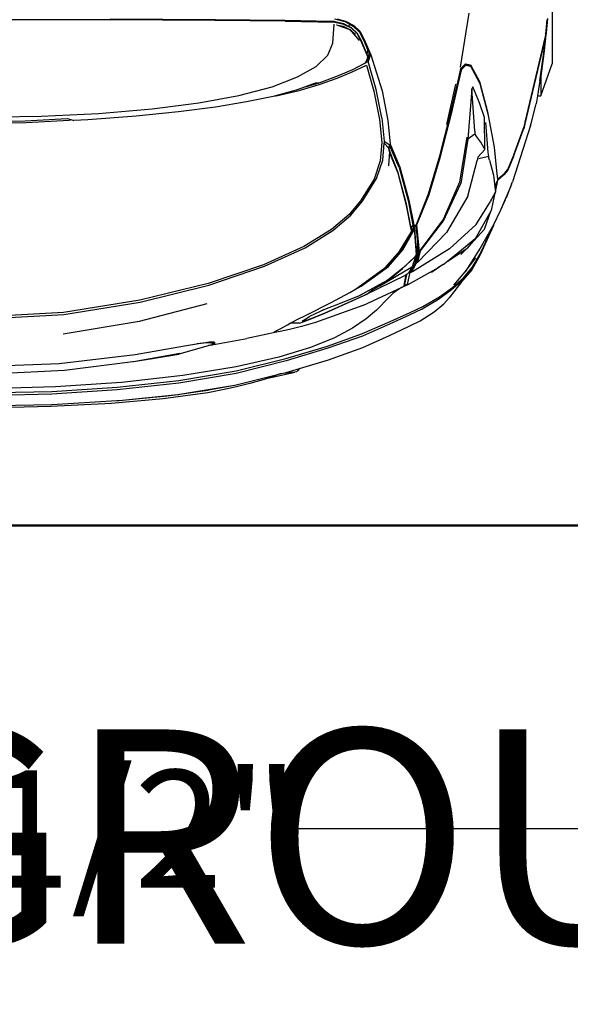
# Model space of a CAD drawing. Units: inches. Extents: x 22042254 to 25404563, y 17568978 to 17626777.
# Tile 23 of 45: x 22179852 to 22179889, y 17626160 to 17626227. Entities that reach past the tile are written whole.
import ezdxf

# ---------------------------------------------------------------- set-up
doc = ezdxf.new("R2010")
doc.units = ezdxf.units.IN
doc.header["$MEASUREMENT"] = 0
for name, color, linetype, lineweight in [('A-ANNO-DIMS', 2, 'Continuous', 18), ('A-SITE-VEHI', 8, 'Continuous', 18), ('text', 7, 'Continuous', 25), ('walls', 252, 'Continuous', 50)]:
    doc.layers.add(name, color=color, linetype=linetype, lineweight=lineweight)
doc.layers.add('Edges', color=250, linetype='Continuous')
doc.styles.get("Standard").update_dxf_attribs({"font": 'arial.ttf'})
doc.dimstyles.get("Standard").update_dxf_attribs({"dimtxt": 8, "dimasz": 0.18, "dimexe": 0.18, "dimexo": 0.0625, "dimgap": 0.09, "dimtad": 0, "dimtih": 1, "dimtoh": 1, "dimzin": 0, "dimdsep": 46, "dimlunit": 3, "dimtxsty": 'Standard', "dimcen": 0.09, "dimadec": 0, "dimazin": 0, "dimtfac": 1, "dimtofl": 0, "dimtmove": 0, "dimatfit": 3, "dimfxl": 1, "dimtolj": 1, "dimtzin": 0, "dimarcsym": 0})

# ---------------------------------------------------------------- blocks, each defined once
blk = doc.blocks.new('Nissan Qashqai pl')
at = {"layer": 'Edges'}
for p, q in [((10.9577, 12.8101), (11.1283, 12.8101)), ((11.0576, 12.8026), (11.0798, 12.8008)), ((11.0768, 12.8008), (11.059, 12.8023)), ((11.0811, 12.8004), (11.0768, 12.8008)), ((11.0798, 12.8008), (11.0872, 12.7999)), ((11.0827, 12.8001), (11.0811, 12.8004)), ((11.0827, 12.8001), (11.0813, 12.7998)), ((11.0836, 12.8002), (11.0827, 12.8001)), ((11.0856, 12.7994), (11.0827, 12.8001)), ((11.0872, 12.7999), (11.0836, 12.8002)), ((11.0836, 12.8002), (11.0882, 12.7992)), ((11.2196, 12.7681), (11.0856, 12.7994)), ((11.0883, 12.7998), (11.0872, 12.7999)), ((11.0882, 12.7992), (11.2222, 12.7676)), ((11.0883, 12.7998), (11.1123, 12.797)), ((11.1147, 12.7965), (11.0883, 12.7998)), ((11.1123, 12.797), (11.1475, 12.7921)), ((11.1547, 12.791), (11.1147, 12.7965)), ((11.1783, 12.7921), (11.1283, 12.8101)), ((11.1475, 12.7921), (11.1525, 12.7914)), ((11.1475, 12.7921), (11.1783, 12.7921)), ((11.1525, 12.7914), (11.1547, 12.791)), ((11.1547, 12.791), (11.1783, 12.787)), ((11.1783, 12.787), (11.1783, 12.7921)), ((11.1783, 12.787), (11.1906, 12.7849)), ((11.1906, 12.7849), (11.1909, 12.7849)), ((11.193, 12.7845), (11.1909, 12.7849)), ((11.2215, 12.7775), (11.193, 12.7845)), ((11.2247, 12.767), (11.2163, 12.7689)), ((11.22, 12.768), (11.2196, 12.7681)), ((11.2247, 12.767), (11.22, 12.768)), ((11.2247, 12.7764), (11.2215, 12.7775)), ((11.2222, 12.7676), (11.2271, 12.7664)), ((11.2247, 12.7764), (11.3124, 12.7479)), ((11.2253, 12.7668), (11.2247, 12.767)), ((11.2304, 12.7649), (11.2253, 12.7668)), ((11.2253, 12.7668), (11.2271, 12.7664)), ((11.2271, 12.7664), (11.2296, 12.7658)), ((11.2271, 12.7664), (11.2277, 12.7662)), ((11.2277, 12.7662), (11.2296, 12.7658)), ((11.2732, 12.7496), (11.2277, 12.7662)), ((11.2704, 12.7504), (11.2304, 12.7649)), ((11.2702, 12.7507), (11.2704, 12.7504)), ((11.2704, 12.7506), (11.2707, 12.7503)), ((11.2707, 12.7503), (11.2704, 12.7504)), ((11.2719, 12.7498), (11.2707, 12.7503)), ((11.2934, 12.741), (11.2719, 12.7498)), ((11.2732, 12.7496), (11.2946, 12.7409)), ((11.3, 12.735), (11.2934, 12.741)), ((11.2946, 12.7409), (11.3018, 12.7346)), ((11.3081, 12.7253), (11.3, 12.735)), ((11.3018, 12.7346), (11.3103, 12.7249)), ((11.3161, 12.7467), (11.3124, 12.7479)), ((11.3161, 12.7467), (11.3376, 12.7381)), ((11.3192, 12.7454), (11.3566, 12.7294)), ((11.3405, 12.7369), (11.3376, 12.7381)), ((11.3405, 12.7369), (11.3566, 12.7294)), ((11.2091, 12.7103), (11.2583, 12.7196)), ((11.2583, 12.7196), (11.2956, 12.7234)), ((11.2956, 12.7234), (11.3085, 12.7247)), ((11.3022, 12.7186), (11.3252, 12.7213)), ((11.3086, 12.7247), (11.3081, 12.7253)), ((11.3081, 12.7253), (11.3087, 12.7247)), ((11.3085, 12.7247), (11.3086, 12.7247)), ((11.3086, 12.7247), (11.3087, 12.7247)), ((11.3087, 12.7247), (11.3103, 12.7249)), ((11.3103, 12.7249), (11.3103, 12.7249)), ((11.3103, 12.7249), (11.3106, 12.7249)), ((11.3106, 12.7249), (11.314, 12.7238)), ((11.317, 12.7227), (11.3119, 12.7236)), ((11.3132, 12.7243), (11.3256, 12.7215)), ((11.314, 12.7238), (11.317, 12.7227)), ((11.314, 12.7238), (11.3242, 12.7216)), ((11.3242, 12.7216), (11.317, 12.7227)), ((11.3198, 12.7211), (11.3252, 12.7213)), ((11.3242, 12.7216), (11.3256, 12.7215)), ((11.3252, 12.7213), (11.3283, 12.7214)), ((11.3256, 12.7215), (11.3283, 12.7214)), ((11.3283, 12.7214), (11.3297, 12.7206)), ((11.3297, 12.7206), (11.3446, 12.7173)), ((11.3297, 12.7206), (11.3302, 12.7203)), ((11.3302, 12.7203), (11.3446, 12.7173)), ((11.3302, 12.7203), (11.3394, 12.7152)), ((11.3566, 12.7294), (11.3796, 12.7187)), ((11.3796, 12.7187), (11.4164, 12.6974)), ((11.3796, 12.7187), (11.3807, 12.7182)), ((11.156, 12.6966), (11.203, 12.7093)), ((11.1589, 12.6971), (11.2062, 12.7098)), ((11.2121, 12.7043), (11.189, 12.6968)), ((11.203, 12.7093), (11.2091, 12.7103)), ((11.2062, 12.7098), (11.2091, 12.7103)), ((11.2622, 12.7051), (11.2121, 12.7043)), ((11.2199, 12.706), (11.2666, 12.7097)), ((11.2601, 12.7037), (11.2505, 12.6987)), ((11.2622, 12.7051), (11.2601, 12.7037)), ((11.2743, 12.6942), (11.2622, 12.7051)), ((11.2666, 12.7097), (11.2729, 12.7104)), ((11.2787, 12.7123), (11.2729, 12.7104)), ((11.2729, 12.7104), (11.2766, 12.6957)), ((11.2787, 12.7123), (11.3022, 12.7186)), ((11.3394, 12.7152), (11.3434, 12.7138)), ((11.3394, 12.7152), (11.342, 12.7137)), ((11.379, 12.6915), (11.3434, 12.7138)), ((11.3446, 12.7173), (11.3571, 12.7146)), ((11.3583, 12.7142), (11.3571, 12.7146)), ((11.3571, 12.7146), (11.3821, 12.7008)), ((11.3583, 12.7142), (11.3821, 12.7008)), ((11.3864, 12.7044), (11.3583, 12.7142)), ((11.3807, 12.7182), (11.4267, 12.6979)), ((11.4228, 12.6989), (11.3807, 12.7182)), ((11.4163, 12.6775), (11.3864, 12.7044)), ((11.1298, 12.6823), (11.156, 12.6966)), ((11.1365, 12.6851), (11.1589, 12.6971)), ((11.189, 12.6968), (11.1644, 12.6862)), ((11.2337, 12.6892), (11.1672, 12.6844)), ((11.2337, 12.6892), (11.2382, 12.6892)), ((11.2382, 12.6892), (11.2401, 12.6908)), ((11.2382, 12.6892), (11.2459, 12.6785)), ((11.2505, 12.6987), (11.2401, 12.6908)), ((11.2743, 12.6942), (11.2791, 12.6927)), ((11.335, 12.6786), (11.2791, 12.6927)), ((11.379, 12.6915), (11.417, 12.6499)), ((11.3821, 12.7008), (11.4014, 12.69)), ((11.4014, 12.69), (11.4022, 12.6894)), ((11.4014, 12.69), (11.4265, 12.6594)), ((11.4022, 12.6894), (11.4163, 12.6775)), ((11.4022, 12.6894), (11.4265, 12.6594)), ((11.4164, 12.6974), (11.4531, 12.6744)), ((11.4243, 12.6982), (11.4228, 12.6989)), ((11.4464, 12.6853), (11.4243, 12.6982)), ((11.4267, 12.6979), (11.4498, 12.6844)), ((11.4531, 12.6744), (11.4314, 12.6911)), ((11.1336, 12.667), (11.0492, 12.6807)), ((11.1285, 12.6745), (11.1298, 12.6823)), ((11.1293, 12.6736), (11.1285, 12.6745)), ((11.1306, 12.6812), (11.1293, 12.6736)), ((11.1353, 12.6677), (11.1293, 12.6736)), ((11.1306, 12.6752), (11.1319, 12.6827)), ((11.1319, 12.6827), (11.1306, 12.6812)), ((11.1347, 12.671), (11.1306, 12.6752)), ((11.1319, 12.6827), (11.1365, 12.6851)), ((11.1644, 12.6862), (11.1672, 12.6844)), ((11.1672, 12.6844), (11.2459, 12.6785)), ((11.2428, 12.6769), (11.3132, 12.6652)), ((11.2459, 12.6785), (11.3153, 12.6672)), ((11.335, 12.6786), (11.3915, 12.6453)), ((11.4366, 12.6471), (11.4163, 12.6775)), ((11.4163, 12.6775), (11.4259, 12.6674)), ((11.4624, 12.6717), (11.4464, 12.6853)), ((11.4498, 12.6844), (11.4662, 12.6706)), ((11.4681, 12.6691), (11.4498, 12.6844)), ((11.4742, 12.6567), (11.4531, 12.6744)), ((11.1366, 12.6691), (11.1347, 12.671)), ((11.1358, 12.6676), (11.1353, 12.6677)), ((11.1358, 12.6676), (11.1366, 12.6691)), ((11.148, 12.665), (11.1358, 12.6676)), ((11.1401, 12.6682), (11.1366, 12.6691)), ((11.2066, 12.6527), (11.1401, 12.6682)), ((11.2063, 12.6515), (11.148, 12.665)), ((11.2232, 12.6458), (11.1598, 12.6594)), ((11.3132, 12.6652), (11.3715, 12.6398)), ((11.3733, 12.6404), (11.3153, 12.6672)), ((11.4265, 12.6594), (11.4366, 12.6471)), ((11.4774, 12.6543), (11.4624, 12.6717)), ((11.4662, 12.6706), (11.4815, 12.6531)), ((11.4681, 12.6691), (11.4936, 12.6491)), ((11.272, 12.6349), (11.2063, 12.6515)), ((11.2728, 12.6357), (11.2066, 12.6527)), ((11.3915, 12.6453), (11.4381, 12.6002)), ((11.417, 12.6499), (11.4529, 12.5922)), ((11.4366, 12.6471), (11.4408, 12.6419)), ((11.4408, 12.6419), (11.4411, 12.6414)), ((11.4924, 12.6339), (11.4774, 12.6543)), ((11.4815, 12.6531), (11.4963, 12.6328)), ((11.4936, 12.6491), (11.5033, 12.6408)), ((11.3311, 12.6172), (11.272, 12.6349)), ((11.3323, 12.6178), (11.2728, 12.6357)), ((11.3715, 12.6398), (11.4177, 12.6052)), ((11.4203, 12.6044), (11.3733, 12.6404)), ((11.4411, 12.6414), (11.4411, 12.6414)), ((11.4414, 12.6409), (11.4411, 12.6414)), ((11.4414, 12.6409), (11.447, 12.6315)), ((11.4455, 12.6336), (11.4414, 12.6409)), ((11.447, 12.6315), (11.4455, 12.6336)), ((11.4455, 12.6336), (11.4462, 12.6324)), ((11.447, 12.6315), (11.4462, 12.6324)), ((11.4732, 12.585), (11.4462, 12.6324)), ((11.447, 12.6315), (11.447, 12.6314)), ((11.4536, 12.6215), (11.447, 12.6314)), ((11.5074, 12.608), (11.4924, 12.6339)), ((11.4964, 12.6326), (11.4963, 12.6328)), ((11.4964, 12.6326), (11.5113, 12.6069)), ((11.5158, 12.6256), (11.5033, 12.6408)), ((11.3751, 12.5999), (11.3311, 12.6172)), ((11.3747, 12.6011), (11.3323, 12.6178)), ((11.5295, 12.6041), (11.5158, 12.6256)), ((11.38, 12.5988), (11.3747, 12.6011)), ((11.3751, 12.5999), (11.3762, 12.5999)), ((11.3752, 12.5998), (11.3751, 12.5999)), ((11.3763, 12.5998), (11.3752, 12.5998)), ((11.3764, 12.5993), (11.3752, 12.5998)), ((11.3792, 12.5982), (11.3764, 12.5993)), ((11.3792, 12.5982), (11.3793, 12.5979)), ((11.3792, 12.5982), (11.3804, 12.5972)), ((11.3853, 12.5993), (11.38, 12.5988)), ((11.3804, 12.5972), (11.4082, 12.5998)), ((11.3827, 12.5953), (11.3804, 12.5972)), ((11.3811, 12.5958), (11.3808, 12.5961)), ((11.3846, 12.5953), (11.4248, 12.5976)), ((11.4212, 12.603), (11.3853, 12.5993)), ((11.3915, 12.5951), (11.4266, 12.5977)), ((11.409, 12.5999), (11.4082, 12.5998)), ((11.4164, 12.5998), (11.4082, 12.5998)), ((11.4152, 12.6004), (11.409, 12.5999)), ((11.409, 12.5999), (11.4163, 12.5999)), ((11.4173, 12.6006), (11.4152, 12.6004)), ((11.4163, 12.5999), (11.4152, 12.6004)), ((11.4163, 12.5999), (11.4186, 12.5999)), ((11.4164, 12.5998), (11.4163, 12.5999)), ((11.4181, 12.5998), (11.4164, 12.5998)), ((11.4169, 12.5996), (11.4164, 12.5998)), ((11.4252, 12.598), (11.4169, 12.5996)), ((11.4176, 12.6007), (11.4173, 12.6006)), ((11.418, 12.6006), (11.4173, 12.6006)), ((11.4215, 12.601), (11.4176, 12.6007)), ((11.418, 12.6006), (11.4176, 12.6007)), ((11.4177, 12.6052), (11.4193, 12.6042)), ((11.4204, 12.6002), (11.418, 12.6006)), ((11.4194, 12.6), (11.418, 12.6006)), ((11.4192, 12.6045), (11.4194, 12.6042)), ((11.4194, 12.6042), (11.4193, 12.6042)), ((11.4193, 12.6042), (11.4196, 12.604)), ((11.4194, 12.6042), (11.4196, 12.604)), ((11.4196, 12.6042), (11.4194, 12.6042)), ((11.4196, 12.604), (11.4201, 12.6036)), ((11.4198, 12.6041), (11.4201, 12.6036)), ((11.4201, 12.6036), (11.4212, 12.603)), ((11.4292, 12.6024), (11.4203, 12.6044)), ((11.4229, 12.6025), (11.4203, 12.6044)), ((11.4212, 12.603), (11.4215, 12.601)), ((11.4218, 12.6028), (11.4212, 12.603)), ((11.4215, 12.601), (11.4219, 12.6009)), ((11.4222, 12.6029), (11.4218, 12.6028)), ((11.4229, 12.6025), (11.4218, 12.6028)), ((11.4219, 12.6009), (11.4222, 12.6005)), ((11.4219, 12.6009), (11.4224, 12.6008)), ((11.4224, 12.6008), (11.4226, 12.6006)), ((11.4224, 12.6008), (11.423, 12.6006)), ((11.4315, 12.6002), (11.4229, 12.6025)), ((11.423, 12.6006), (11.4229, 12.6025)), ((11.44, 12.5959), (11.423, 12.6006)), ((11.4248, 12.5976), (11.4266, 12.5977)), ((11.4266, 12.5977), (11.4252, 12.598)), ((11.4266, 12.5977), (11.4268, 12.5977)), ((11.4268, 12.5977), (11.4296, 12.5954)), ((11.4268, 12.5977), (11.4278, 12.5977)), ((11.4303, 12.5956), (11.4278, 12.5977)), ((11.4278, 12.5977), (11.43, 12.5969)), ((11.4381, 12.6002), (11.4292, 12.6024)), ((11.4337, 12.5962), (11.43, 12.5969)), ((11.43, 12.5969), (11.4361, 12.5948)), ((11.4403, 12.5978), (11.4315, 12.6002)), ((11.4397, 12.5937), (11.4337, 12.5962)), ((11.4381, 12.6002), (11.4403, 12.5978)), ((11.4403, 12.5978), (11.44, 12.5959)), ((11.44, 12.5959), (11.4457, 12.5928)), ((11.4462, 12.5947), (11.4403, 12.5978)), ((11.5165, 12.5882), (11.5074, 12.608)), ((11.5113, 12.6068), (11.5113, 12.6069)), ((11.5113, 12.6068), (11.5206, 12.5869)), ((11.5384, 12.5859), (11.5295, 12.6041)), ((11.2895, 12.5724), (11.3411, 12.5863)), ((11.29, 12.5711), (11.3419, 12.585)), ((11.3474, 12.5827), (11.2972, 12.5692)), ((11.3493, 12.5828), (11.2993, 12.5695)), ((11.3411, 12.5863), (11.3795, 12.5939)), ((11.3419, 12.585), (11.3804, 12.5926)), ((11.3847, 12.5899), (11.3474, 12.5827)), ((11.3474, 12.5827), (11.3474, 12.5827)), ((11.3863, 12.5898), (11.3493, 12.5828)), ((11.3795, 12.5939), (11.3834, 12.5947)), ((11.3804, 12.5926), (11.3841, 12.5933)), ((11.3847, 12.5899), (11.3804, 12.5926)), ((11.3834, 12.5947), (11.3827, 12.5953)), ((11.3846, 12.5953), (11.3829, 12.5952)), ((11.3829, 12.5952), (11.3849, 12.5951)), ((11.388, 12.591), (11.3829, 12.5952)), ((11.3834, 12.5947), (11.3841, 12.5933)), ((11.3846, 12.5953), (11.3846, 12.5953)), ((11.3851, 12.5951), (11.3846, 12.5953)), ((11.3846, 12.5953), (11.3849, 12.5951)), ((11.3847, 12.5899), (11.3848, 12.5899)), ((11.388, 12.591), (11.3848, 12.5899)), ((11.3849, 12.5951), (11.3851, 12.5951)), ((11.3882, 12.5923), (11.3849, 12.5951)), ((11.3851, 12.5951), (11.3867, 12.5949)), ((11.4171, 12.5766), (11.3851, 12.5951)), ((11.3895, 12.5912), (11.3863, 12.5898)), ((11.3867, 12.5949), (11.3915, 12.5951)), ((11.3914, 12.5926), (11.3867, 12.5949)), ((11.3886, 12.5919), (11.3872, 12.5927)), ((11.3882, 12.5923), (11.3886, 12.5919)), ((11.3886, 12.5919), (11.3895, 12.5912)), ((11.3892, 12.5916), (11.3886, 12.5919)), ((11.3923, 12.5894), (11.3895, 12.5912)), ((11.4187, 12.5768), (11.3914, 12.5926)), ((11.4203, 12.5724), (11.3923, 12.5894)), ((11.4296, 12.5954), (11.4469, 12.5773)), ((11.4479, 12.5766), (11.4303, 12.5956)), ((11.4361, 12.5948), (11.4406, 12.5932)), ((11.4406, 12.5932), (11.4397, 12.5937)), ((11.4406, 12.5932), (11.4442, 12.592)), ((11.4442, 12.592), (11.4497, 12.589)), ((11.4462, 12.5893), (11.4442, 12.592)), ((11.4457, 12.5928), (11.4512, 12.5893)), ((11.452, 12.591), (11.4462, 12.5947)), ((11.475, 12.5409), (11.4462, 12.5893)), ((11.4497, 12.589), (11.4498, 12.5889)), ((11.4535, 12.5876), (11.4498, 12.5889)), ((11.4498, 12.5889), (11.4549, 12.5855)), ((11.4512, 12.5893), (11.4535, 12.5876)), ((11.4539, 12.5897), (11.452, 12.591)), ((11.4529, 12.5922), (11.4542, 12.5894)), ((11.4535, 12.5876), (11.4532, 12.5882)), ((11.4535, 12.5876), (11.4542, 12.5894)), ((11.4535, 12.5876), (11.4728, 12.5838)), ((11.4542, 12.5894), (11.4539, 12.5897)), ((11.4549, 12.5855), (11.4568, 12.5836)), ((11.4564, 12.5833), (11.4567, 12.5833)), ((11.4569, 12.583), (11.4565, 12.5831)), ((11.4568, 12.5836), (11.4571, 12.5833)), ((11.4571, 12.5833), (11.4573, 12.583)), ((11.4573, 12.583), (11.4578, 12.5822)), ((11.4704, 12.5803), (11.4573, 12.583)), ((11.4573, 12.5823), (11.4574, 12.5822)), ((11.4573, 12.5823), (11.4573, 12.5823)), ((11.4576, 12.5822), (11.4574, 12.5822)), ((11.4578, 12.5822), (11.4588, 12.5807)), ((11.4605, 12.5816), (11.4578, 12.5822)), ((11.4588, 12.5807), (11.4895, 12.5178)), ((11.4713, 12.5794), (11.4605, 12.5816)), ((11.4742, 12.5797), (11.4704, 12.5803)), ((11.4732, 12.585), (11.4728, 12.5838)), ((11.4728, 12.5838), (11.4742, 12.5797)), ((11.4728, 12.5838), (11.4746, 12.5796)), ((11.4758, 12.5791), (11.4732, 12.585)), ((11.5306, 12.5573), (11.5165, 12.5882)), ((11.5206, 12.5869), (11.5349, 12.5559)), ((11.5527, 12.5559), (11.5384, 12.5859)), ((11.29, 12.5711), (11.2541, 12.5557)), ((11.2586, 12.5591), (11.2895, 12.5724)), ((11.2972, 12.5692), (11.2677, 12.5575)), ((11.2993, 12.5695), (11.2705, 12.5579)), ((11.4433, 12.5543), (11.4171, 12.5766)), ((11.4447, 12.5545), (11.4187, 12.5768)), ((11.4467, 12.5488), (11.4203, 12.5724)), ((11.4469, 12.5773), (11.4659, 12.5539)), ((11.4654, 12.5548), (11.4479, 12.5766)), ((11.4744, 12.5792), (11.4713, 12.5794)), ((11.4742, 12.5797), (11.4744, 12.5792)), ((11.4745, 12.5797), (11.4742, 12.5797)), ((11.4745, 12.5792), (11.4744, 12.5792)), ((11.4745, 12.5792), (11.4745, 12.5797)), ((11.4745, 12.5797), (11.4746, 12.5796)), ((11.4748, 12.5792), (11.4745, 12.5792)), ((11.4746, 12.5796), (11.4748, 12.5792)), ((11.4746, 12.5796), (11.4758, 12.5791)), ((11.4758, 12.5791), (11.4748, 12.5792)), ((11.4758, 12.5791), (11.4759, 12.579)), ((11.4759, 12.579), (11.4778, 12.5746)), ((11.4759, 12.579), (11.4771, 12.576)), ((11.5057, 12.5145), (11.4771, 12.576)), ((11.4778, 12.5746), (11.4826, 12.5669)), ((11.4826, 12.5669), (11.4869, 12.5615)), ((11.1702, 12.5444), (11.2166, 12.5534)), ((11.2166, 12.5534), (11.2538, 12.5571)), ((11.2488, 12.548), (11.2541, 12.5557)), ((11.2599, 12.5552), (11.2524, 12.5477)), ((11.2538, 12.5571), (11.2586, 12.5591)), ((11.2541, 12.5557), (11.2599, 12.5552)), ((11.2677, 12.5575), (11.2599, 12.5552)), ((11.265, 12.5563), (11.2599, 12.5552)), ((11.2705, 12.5579), (11.265, 12.5563)), ((11.265, 12.5563), (11.2724, 12.5557)), ((11.2724, 12.5557), (11.2874, 12.5544)), ((11.4745, 12.5116), (11.4433, 12.5543)), ((11.4758, 12.5118), (11.4447, 12.5545)), ((11.4633, 12.5594), (11.4897, 12.5108)), ((11.4654, 12.5548), (11.4659, 12.5539)), ((11.4659, 12.5539), (11.4674, 12.5512)), ((11.4675, 12.551), (11.4674, 12.5512)), ((11.4675, 12.551), (11.4703, 12.546)), ((11.4869, 12.5615), (11.4933, 12.555)), ((11.5131, 12.5356), (11.4933, 12.555)), ((11.5496, 12.5141), (11.5306, 12.5573)), ((11.5349, 12.5559), (11.5535, 12.5139)), ((11.5716, 12.5145), (11.5527, 12.5559)), ((11.1144, 12.5271), (11.1702, 12.5444)), ((11.1683, 12.5354), (11.1244, 12.5227)), ((11.2127, 12.5443), (11.1683, 12.5354)), ((11.1712, 12.5317), (11.2152, 12.5404)), ((11.2127, 12.5443), (11.2488, 12.548)), ((11.2152, 12.5404), (11.2509, 12.5439)), ((11.2488, 12.548), (11.2524, 12.5477)), ((11.2509, 12.5439), (11.28, 12.5414)), ((11.2785, 12.5455), (11.2524, 12.5477)), ((11.3076, 12.5358), (11.2785, 12.5455)), ((11.28, 12.5414), (11.3082, 12.532)), ((11.3428, 12.5139), (11.3076, 12.5358)), ((11.4801, 12.503), (11.4467, 12.5488)), ((11.4703, 12.546), (11.4704, 12.5458)), ((11.4704, 12.5458), (11.4909, 12.5085)), ((11.4704, 12.5458), (11.4897, 12.5108)), ((11.475, 12.5409), (11.4828, 12.5276)), ((11.5131, 12.5356), (11.5265, 12.5194)), ((11.0902, 12.5166), (11.1144, 12.5271)), ((11.0908, 12.5153), (11.107, 12.5224)), ((11.1138, 12.5213), (11.0912, 12.5117)), ((11.1149, 12.5212), (11.0917, 12.5114)), ((11.107, 12.5224), (11.1116, 12.5243)), ((11.1138, 12.5213), (11.107, 12.5224)), ((11.1116, 12.5243), (11.1147, 12.5257)), ((11.1244, 12.5227), (11.1116, 12.5243)), ((11.1139, 12.5213), (11.1138, 12.5213)), ((11.1164, 12.5224), (11.1139, 12.5213)), ((11.1147, 12.5257), (11.1244, 12.5227)), ((11.1172, 12.5222), (11.1149, 12.5212)), ((11.1164, 12.5224), (11.1174, 12.5223)), ((11.1173, 12.5222), (11.1172, 12.5222)), ((11.1174, 12.5223), (11.1173, 12.5222)), ((11.12, 12.5215), (11.1174, 12.5223)), ((11.1246, 12.5199), (11.12, 12.5215)), ((11.1259, 12.5194), (11.1244, 12.5227)), ((11.1244, 12.5227), (11.126, 12.5194)), ((11.1259, 12.5194), (11.1246, 12.5199)), ((11.126, 12.5193), (11.1247, 12.5197)), ((11.126, 12.5193), (11.1248, 12.5195)), ((11.1251, 12.5189), (11.126, 12.5193)), ((11.126, 12.5193), (11.1259, 12.5194)), ((11.126, 12.5194), (11.1259, 12.5194)), ((11.126, 12.5194), (11.1261, 12.5193)), ((11.1264, 12.5192), (11.126, 12.5194)), ((11.1263, 12.5186), (11.126, 12.5193)), ((11.1261, 12.5193), (11.126, 12.5193)), ((11.1261, 12.5193), (11.1263, 12.5188)), ((11.1264, 12.5192), (11.1261, 12.5193)), ((11.1277, 12.5167), (11.1264, 12.5192)), ((11.1302, 12.52), (11.1712, 12.5317)), ((11.1412, 12.4969), (11.1302, 12.52)), ((11.3082, 12.532), (11.3425, 12.5106)), ((11.488, 12.5208), (11.4828, 12.5276)), ((11.5179, 12.4551), (11.488, 12.5208)), ((11.5265, 12.5194), (11.541, 12.4982)), ((11.0682, 12.5004), (11.0779, 12.5103)), ((11.0692, 12.4996), (11.0787, 12.5092)), ((11.0802, 12.5057), (11.0718, 12.4967)), ((11.0809, 12.5056), (11.0727, 12.4966)), ((11.0747, 12.4944), (11.092, 12.5087)), ((11.0779, 12.5103), (11.0902, 12.5166)), ((11.0787, 12.5092), (11.0908, 12.5153)), ((11.0912, 12.5117), (11.0802, 12.5057)), ((11.0917, 12.5114), (11.0809, 12.5056)), ((11.1369, 12.4986), (11.1277, 12.5167)), ((11.3425, 12.5106), (11.3635, 12.4929)), ((11.3645, 12.4958), (11.3428, 12.5139)), ((11.4788, 12.5052), (11.4745, 12.5116)), ((11.4852, 12.494), (11.4758, 12.5118)), ((11.4801, 12.503), (11.4788, 12.5052)), ((11.4898, 12.5172), (11.4895, 12.5178)), ((11.4897, 12.5108), (11.4909, 12.5085)), ((11.4898, 12.5172), (11.49, 12.5167)), ((11.49, 12.5167), (11.5179, 12.4551)), ((11.4909, 12.5085), (11.5028, 12.4792)), ((11.5057, 12.5145), (11.5325, 12.4404)), ((11.5691, 12.4592), (11.5496, 12.5141)), ((11.5535, 12.5139), (11.5726, 12.46)), ((11.5908, 12.4606), (11.5716, 12.5145)), ((11.0614, 12.4872), (11.0682, 12.5004)), ((11.0624, 12.4866), (11.0658, 12.4932)), ((11.0658, 12.4932), (11.0692, 12.4996)), ((11.0658, 12.4932), (11.0698, 12.4925)), ((11.0698, 12.4925), (11.0659, 12.4848)), ((11.0727, 12.4966), (11.0669, 12.4849)), ((11.0671, 12.4731), (11.0747, 12.4944)), ((11.0696, 12.4836), (11.0747, 12.4944)), ((11.0718, 12.4967), (11.0698, 12.4925)), ((11.0747, 12.4944), (11.0821, 12.5029)), ((11.1475, 12.4741), (11.1369, 12.4986)), ((11.1505, 12.4742), (11.1412, 12.4969)), ((11.3635, 12.4929), (11.3872, 12.4654)), ((11.3888, 12.4678), (11.3645, 12.4958)), ((11.4852, 12.494), (11.4801, 12.503)), ((11.5013, 12.4651), (11.4852, 12.494)), ((11.541, 12.4982), (11.5562, 12.4701)), ((11.0581, 12.4738), (11.0614, 12.4872)), ((11.0582, 12.47), (11.0624, 12.4866)), ((11.063, 12.4728), (11.0622, 12.4697)), ((11.0659, 12.4848), (11.063, 12.4728)), ((11.0641, 12.4733), (11.0632, 12.47)), ((11.0669, 12.4849), (11.0641, 12.4733)), ((11.0671, 12.4731), (11.0696, 12.4836)), ((11.1577, 12.4465), (11.1475, 12.4741)), ((11.1605, 12.4465), (11.1505, 12.4742)), ((11.5028, 12.4792), (11.5118, 12.4548)), ((11.0621, 12.4657), (11.0607, 12.3933)), ((11.0618, 12.3933), (11.0632, 12.47)), ((11.0622, 12.4697), (11.0621, 12.4657)), ((11.0962, 12.4675), (11.0662, 12.4698)), ((11.1148, 12.4598), (11.0962, 12.4675)), ((11.1323, 12.4415), (11.1148, 12.4598)), ((11.3872, 12.4654), (11.4138, 12.4223)), ((11.4159, 12.4242), (11.3888, 12.4678)), ((11.5202, 12.427), (11.5013, 12.4651)), ((11.5562, 12.4701), (11.5715, 12.4326)), ((11.5884, 12.3943), (11.5691, 12.4592)), ((11.5726, 12.46), (11.5922, 12.3947)), ((11.6042, 12.4156), (11.5908, 12.4606)), ((11.1643, 12.425), (11.1576, 12.4459)), ((11.1643, 12.425), (11.1577, 12.4465)), ((11.1583, 12.4423), (11.1643, 12.425)), ((11.1699, 12.4153), (11.1605, 12.4465)), ((11.5118, 12.4548), (11.523, 12.4311)), ((11.5118, 12.4548), (11.513, 12.4514)), ((11.5292, 12.4272), (11.5179, 12.4551)), ((11.5179, 12.4551), (11.5285, 12.4279)), ((11.1487, 12.4126), (11.1323, 12.4415)), ((11.1582, 12.4416), (11.1668, 12.4177)), ((11.5283, 12.4109), (11.5202, 12.427)), ((11.5301, 12.4198), (11.523, 12.4311)), ((11.5285, 12.4279), (11.5302, 12.4209)), ((11.5331, 12.4157), (11.5292, 12.4272)), ((11.5325, 12.4404), (11.5386, 12.4187)), ((11.5715, 12.4326), (11.5866, 12.3835)), ((11.164, 12.373), (11.1487, 12.4126)), ((11.1643, 12.425), (11.1668, 12.4177)), ((11.1668, 12.4177), (11.1694, 12.4104)), ((11.178, 12.379), (11.1699, 12.4153)), ((11.4138, 12.4223), (11.4422, 12.3594)), ((11.4445, 12.3608), (11.4159, 12.4242)), ((11.5302, 12.4209), (11.5301, 12.4198)), ((11.5331, 12.4157), (11.5335, 12.401)), ((11.5386, 12.4187), (11.5434, 12.3997)), ((11.6042, 12.4156), (11.6077, 12.4125)), ((11.6103, 12.395), (11.6042, 12.4156)), ((11.6077, 12.4125), (11.6094, 12.4107)), ((11.1694, 12.4104), (11.1781, 12.3782)), ((11.5334, 12.4014), (11.5283, 12.4109)), ((11.5326, 12.4045), (11.5333, 12.4019)), ((11.5333, 12.4019), (11.5334, 12.4014)), ((11.5335, 12.401), (11.5334, 12.4014)), ((11.5357, 12.3968), (11.5335, 12.401)), ((11.5416, 12.3863), (11.5357, 12.3968)), ((11.5434, 12.3997), (11.5461, 12.3854)), ((11.6094, 12.4107), (11.6101, 12.4085)), ((11.6101, 12.4085), (11.6127, 12.3852)), ((11.6185, 12.3689), (11.6101, 12.4085)), ((11.0607, 12.3933), (11.0595, 12.2842)), ((11.0618, 12.3933), (11.0606, 12.2841)), ((11.5455, 12.3793), (11.5416, 12.3863)), ((11.5461, 12.3854), (11.5467, 12.3822)), ((11.5467, 12.3822), (11.5571, 12.3331)), ((11.5866, 12.3835), (11.6016, 12.3166)), ((11.6076, 12.3166), (11.5884, 12.3943)), ((11.5922, 12.3947), (11.6118, 12.3165)), ((11.6127, 12.3852), (11.6103, 12.395)), ((11.6127, 12.3852), (11.6174, 12.3722)), ((11.6297, 12.3166), (11.6127, 12.3852)), ((11.1776, 12.3211), (11.164, 12.373)), ((11.1781, 12.3782), (11.178, 12.379)), ((11.1781, 12.3782), (11.1791, 12.3746)), ((11.1791, 12.3746), (11.1877, 12.333)), ((11.5472, 12.3757), (11.5455, 12.3793)), ((11.6174, 12.3722), (11.6185, 12.3689)), ((11.6185, 12.3689), (11.6224, 12.3567)), ((11.4422, 12.3594), (11.4712, 12.2729)), ((11.4738, 12.274), (11.4445, 12.3608)), ((11.6224, 12.3567), (11.6277, 12.3379)), ((11.6277, 12.3379), (11.6328, 12.3174)), ((11.1891, 12.2586), (11.1776, 12.3211)), ((11.1877, 12.333), (11.1958, 12.2844)), ((11.5668, 12.2816), (11.5571, 12.3331)), ((11.6016, 12.3166), (11.615, 12.2333)), ((11.6229, 12.2274), (11.6076, 12.3166)), ((11.6118, 12.3165), (11.6272, 12.2272)), ((11.6301, 12.3141), (11.6297, 12.3166)), ((11.6377, 12.2734), (11.6301, 12.3141)), ((11.6332, 12.2951), (11.6301, 12.3141)), ((11.6328, 12.3174), (11.6375, 12.2956)), ((11.6334, 12.2946), (11.6332, 12.2951)), ((11.6443, 12.2288), (11.6334, 12.2946)), ((11.6375, 12.2956), (11.6422, 12.2725)), ((11.0595, 12.2842), (11.0586, 12.1198)), ((11.0606, 12.2841), (11.0597, 12.1196)), ((11.1958, 12.2844), (11.2033, 12.2269)), ((11.4712, 12.2729), (11.4976, 12.1662)), ((11.5005, 12.167), (11.4738, 12.274)), ((11.5626, 12.2771), (11.5627, 12.2817)), ((11.5627, 12.2746), (11.5626, 12.2771)), ((11.5626, 12.2745), (11.5627, 12.2746)), ((11.5627, 12.2817), (11.5634, 12.2829)), ((11.5627, 12.2817), (11.5633, 12.2814)), ((11.5628, 12.2721), (11.5627, 12.2746)), ((11.5632, 12.2783), (11.5633, 12.2814)), ((11.5636, 12.2706), (11.5632, 12.2783)), ((11.5633, 12.2814), (11.5634, 12.2829)), ((11.5633, 12.2814), (11.5661, 12.2803)), ((11.5634, 12.2829), (11.5668, 12.2816)), ((11.5639, 12.2809), (11.5637, 12.2764)), ((11.5637, 12.2763), (11.5637, 12.2764)), ((11.5637, 12.2764), (11.5638, 12.2762)), ((11.5638, 12.2762), (11.5641, 12.2688)), ((11.5643, 12.2808), (11.5639, 12.2809)), ((11.5642, 12.2771), (11.5646, 12.2778)), ((11.566, 12.2801), (11.5643, 12.2808)), ((11.5647, 12.278), (11.5649, 12.2783)), ((11.566, 12.2846), (11.5668, 12.2816)), ((11.566, 12.2801), (11.5661, 12.2803)), ((11.5662, 12.28), (11.566, 12.2801)), ((11.5661, 12.2803), (11.5662, 12.28)), ((11.5662, 12.28), (11.5661, 12.2803)), ((11.5669, 12.2797), (11.5661, 12.2803)), ((11.5669, 12.2797), (11.5662, 12.28)), ((11.5662, 12.28), (11.5662, 12.28)), ((11.5667, 12.2813), (11.567, 12.2796)), ((11.5668, 12.2816), (11.5672, 12.2796)), ((11.567, 12.2796), (11.5669, 12.2797)), ((11.5672, 12.2796), (11.567, 12.2796)), ((11.5678, 12.2766), (11.5672, 12.2796)), ((11.5673, 12.2784), (11.5677, 12.2767)), ((11.5678, 12.2766), (11.5818, 12.227)), ((11.5682, 12.2743), (11.5682, 12.2742)), ((11.5683, 12.2739), (11.5683, 12.2739)), ((11.5683, 12.2738), (11.5683, 12.2737)), ((11.6378, 12.2728), (11.6377, 12.2734)), ((11.6381, 12.2716), (11.6378, 12.2728)), ((11.639, 12.2645), (11.6378, 12.2728)), ((11.1984, 12.1855), (11.1891, 12.2586)), ((11.5033, 12.271), (11.5307, 12.165)), ((11.565, 12.2577), (11.5636, 12.2706)), ((11.5641, 12.2688), (11.5656, 12.2559)), ((11.5685, 12.2359), (11.565, 12.2577)), ((11.639, 12.2645), (11.6381, 12.2716)), ((11.6443, 12.2288), (11.639, 12.2645)), ((11.6422, 12.2725), (11.6514, 12.2026)), ((11.2033, 12.2269), (11.21, 12.1607)), ((11.5823, 12.1589), (11.5685, 12.2359)), ((11.593, 12.1566), (11.58, 12.2288)), ((11.5883, 12.186), (11.5816, 12.2272)), ((11.5883, 12.186), (11.5818, 12.227)), ((11.615, 12.2333), (11.626, 12.1375)), ((11.6333, 12.131), (11.6229, 12.2274)), ((11.6272, 12.2272), (11.6377, 12.1308)), ((11.6446, 12.2271), (11.6443, 12.2288)), ((11.6448, 12.2258), (11.6446, 12.2271)), ((11.6474, 12.2042), (11.6448, 12.2258)), ((11.6539, 12.1338), (11.6448, 12.2258)), ((11.6474, 12.2038), (11.6474, 12.2042)), ((11.6475, 12.2032), (11.6474, 12.2038)), ((11.648, 12.198), (11.6475, 12.2032)), ((11.6539, 12.1338), (11.648, 12.198)), ((11.6514, 12.2026), (11.6589, 12.1222)), ((11.2057, 12.1019), (11.1984, 12.1855)), ((11.593, 12.1566), (11.5883, 12.186)), ((11.4976, 12.1662), (11.5166, 12.0471)), ((11.5196, 12.0475), (11.5005, 12.167)), ((11.21, 12.1607), (11.2159, 12.085)), ((11.5307, 12.165), (11.5504, 12.0466)), ((11.5963, 12.0406), (11.5823, 12.1589)), ((11.5932, 12.1556), (11.593, 12.1566)), ((11.6067, 12.0489), (11.5932, 12.1556)), ((11.626, 12.1375), (11.6329, 12.0344)), ((11.0597, 12.1196), (11.0594, 11.9221)), ((11.6399, 12.029), (11.6333, 12.131)), ((11.6377, 12.1308), (11.6444, 12.0289)), ((11.6543, 12.1306), (11.6539, 12.1338)), ((11.6604, 12.0287), (11.6543, 12.1306)), ((11.6589, 12.1222), (11.6635, 12.0274)), ((11.2101, 12.012), (11.2057, 12.1019)), ((11.2159, 12.085), (11.2166, 12.063)), ((11.2139, 12.0528), (11.2158, 12.0599)), ((11.2158, 12.0602), (11.2166, 12.063)), ((11.2158, 12.0602), (11.2168, 12.056)), ((11.2158, 12.0599), (11.2158, 12.0602)), ((11.2158, 12.0599), (11.2168, 12.056)), ((11.2174, 11.9874), (11.2139, 12.0528)), ((11.2168, 12.056), (11.2204, 11.989)), ((11.5166, 12.0471), (11.5239, 11.9221)), ((11.527, 11.9221), (11.5196, 12.0475)), ((11.6133, 11.9221), (11.6067, 12.0489)), ((11.6005, 11.9335), (11.5963, 12.0406)), ((11.6329, 12.0344), (11.6363, 11.9221)), ((11.6421, 11.9221), (11.6399, 12.029)), ((11.6444, 12.0289), (11.6465, 11.9221)), ((11.6623, 11.9221), (11.6604, 12.0287)), ((11.6635, 12.0274), (11.6663, 11.9221)), ((11.2116, 11.9221), (11.2101, 12.012)), ((11.218, 11.9221), (11.2174, 11.9874)), ((11.2204, 11.989), (11.2211, 11.9221))]:
    blk.add_line(p, q, dxfattribs=at)
blk = doc.blocks.new('CAR')
blk.add_blockref('Nissan Qashqai pl', (-9.7433, -11.9151))
blk = doc.blocks.new('*D59')
at = {"layer": 'A-ANNO-DIMS', "color": 0, "lineweight": -2, "transparency": 16777216}
for p, q in [((22179802.402, 17626200.497), (22179802.402, 17626171.756)), ((22179895.926, 17626200.497), (22179895.926, 17626171.756)), ((22179802.582, 17626171.936), (22179829.153, 17626171.936)), ((22179895.746, 17626171.936), (22179869.175, 17626171.936))]:
    blk.add_line(p, q, dxfattribs=at)
at = {"layer": 'A-ANNO-DIMS', "color": 0, "transparency": 16777216}
for points in [[(22179802.582, 17626171.966), (22179802.582, 17626171.906), (22179802.402, 17626171.936)], [(22179895.746, 17626171.966), (22179895.746, 17626171.906), (22179895.926, 17626171.936)]]:
    blk.add_solid(points, dxfattribs=at)
at = {"layer": 'Defpoints', "color": 0, "transparency": 16777216}
for p in [(22179802.402, 17626200.559), (22179895.926, 17626200.559), (22179895.926, 17626171.936)]:
    blk.add_point(p, dxfattribs=at)
at = {"layer": 'A-ANNO-DIMS', "color": 0, "transparency": 16777216, "insert": (22179849.164, 17626171.936), "char_height": 8, "attachment_point": 5}
blk.add_mtext('\\A1;7\'-9 1/2"', dxfattribs=at)

msp = doc.modelspace()

# ---------------------------------------------------------------- linework, layer by layer
at = {"layer": 'walls'}
msp.add_line((22179783.734, 17626192.584), (22179936.734, 17626192.584), dxfattribs=at)

# ---------------------------------------------------------------- block references
at = {"layer": 'A-SITE-VEHI', "xscale": 43.56002006885659, "yscale": 43.56002006885659, "zscale": 43.56002006885659, "rotation": 270}
msp.add_blockref('CAR', (22179848.861, 17626284.325), dxfattribs=at)

# ---------------------------------------------------------------- texts
at = {"layer": 'text'}
msp.add_text('GROUND FLOOR PLAN', height=14.58777, dxfattribs=at).set_placement((22179841.196, 17626164.124))

# ---------------------------------------------------------------- dimensions: what is measured, and where the dimension line sits
at = {"layer": 'A-ANNO-DIMS'}
dim = msp.add_linear_dim(base=(22179895.926, 17626171.936), p1=(22179802.402, 17626200.559), p2=(22179895.926, 17626200.559), dimstyle='Standard', override={"dimdec": 1, "dimlfac": 1, "dimrnd": 0, "dimzin": 1, "dimdsep": 46, "dimlunit": 4, "dimfrac": 2}, dxfattribs=at)
dim.commit()
dim.dimension.update_dxf_attribs({"geometry": '*D59', "text_midpoint": (22179849.164, 17626171.936)})

doc.saveas('drawing.dxf')
